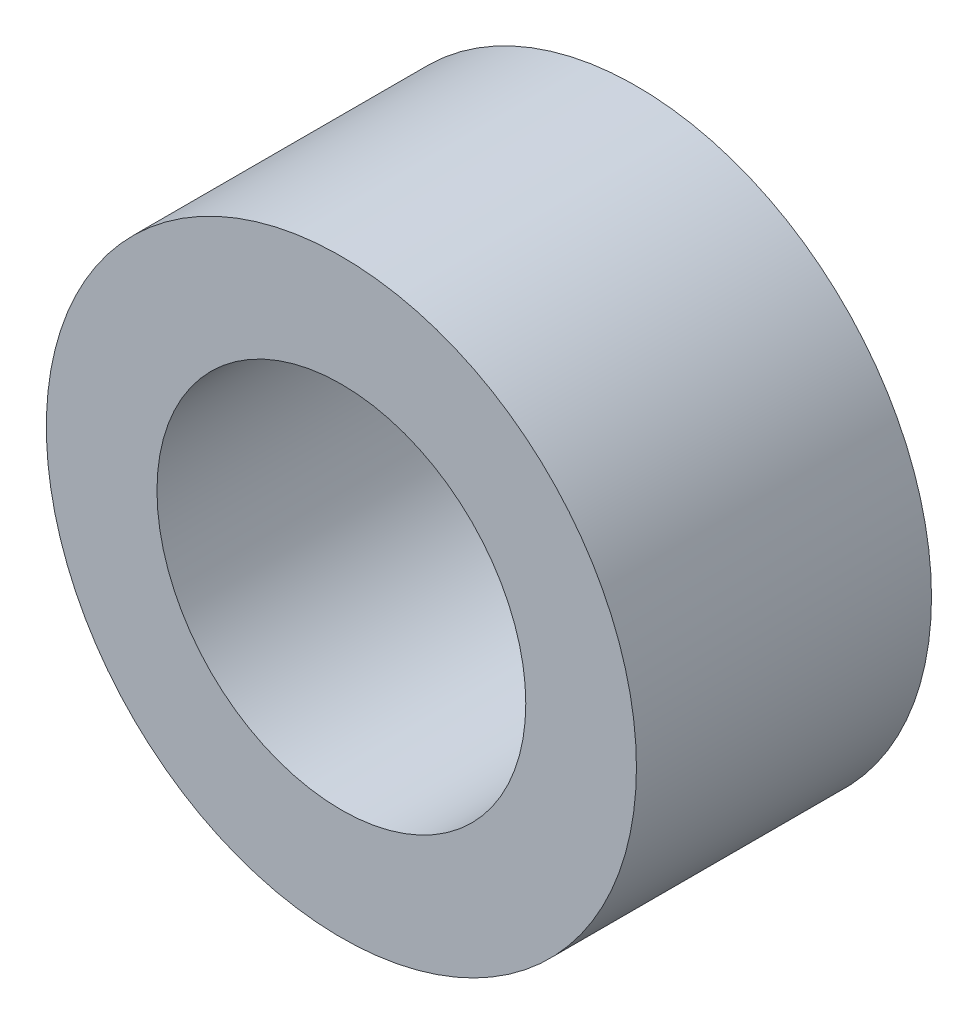
ISO-10303-21;
HEADER;
FILE_DESCRIPTION(('STEP AP214'),'2;1');
FILE_NAME('part.step','',(''),(''),'','','');
FILE_SCHEMA(('AUTOMOTIVE_DESIGN { 1 0 10303 214 1 1 1 1 }'));
ENDSEC;
DATA;
#1=APPLICATION_CONTEXT('core data for automotive mechanical design processes');
#2=APPLICATION_PROTOCOL_DEFINITION('international standard','automotive_design',2000,#1);
#3=PRODUCT_CONTEXT('',#1,'mechanical');
#4=PRODUCT('Part','Part','',(#3));
#5=PRODUCT_RELATED_PRODUCT_CATEGORY('part','',(#4));
#6=PRODUCT_DEFINITION_FORMATION('','',#4);
#7=PRODUCT_DEFINITION_CONTEXT('part definition',#1,'design');
#8=PRODUCT_DEFINITION('design','',#6,#7);
#9=PRODUCT_DEFINITION_SHAPE('','',#8);
#10=(LENGTH_UNIT() NAMED_UNIT(*) SI_UNIT(.MILLI.,.METRE.));
#11=(NAMED_UNIT(*) PLANE_ANGLE_UNIT() SI_UNIT($,.RADIAN.));
#12=(NAMED_UNIT(*) SI_UNIT($,.STERADIAN.) SOLID_ANGLE_UNIT());
#13=UNCERTAINTY_MEASURE_WITH_UNIT(LENGTH_MEASURE(1.E-05),#10,'distance_accuracy_value','');
#14=(GEOMETRIC_REPRESENTATION_CONTEXT(3) GLOBAL_UNCERTAINTY_ASSIGNED_CONTEXT((#13)) GLOBAL_UNIT_ASSIGNED_CONTEXT((#10,
#11,#12)) REPRESENTATION_CONTEXT('',''));
#15=CARTESIAN_POINT('',(0.,0.,0.));
#16=DIRECTION('',(0.,0.,1.));
#17=DIRECTION('',(1.,0.,0.));
#18=AXIS2_PLACEMENT_3D('',#15,#16,#17);
#19=CARTESIAN_POINT('',(0.,0.,2.5));
#20=DIRECTION('',(0.,0.,1.));
#21=DIRECTION('',(1.,0.,0.));
#22=AXIS2_PLACEMENT_3D('',#19,#20,#21);
#23=PLANE('',#22);
#24=CARTESIAN_POINT('',(0.,0.,2.5));
#25=DIRECTION('',(0.,0.,1.));
#26=DIRECTION('',(1.,0.,0.));
#27=AXIS2_PLACEMENT_3D('',#24,#25,#26);
#28=CIRCLE('',#27,5.);
#29=CARTESIAN_POINT('',(5.,0.,2.5));
#30=VERTEX_POINT('',#29);
#31=EDGE_CURVE('E10',#30,#30,#28,.T.);
#32=ORIENTED_EDGE('',*,*,#31,.T.);
#33=EDGE_LOOP('',(#32));
#34=FACE_BOUND('',#33,.T.);
#35=CARTESIAN_POINT('',(0.,0.,2.5));
#36=DIRECTION('',(0.,0.,1.));
#37=DIRECTION('',(1.,0.,0.));
#38=AXIS2_PLACEMENT_3D('',#35,#36,#37);
#39=CIRCLE('',#38,3.125);
#40=CARTESIAN_POINT('',(3.125,0.,2.5));
#41=VERTEX_POINT('',#40);
#42=EDGE_CURVE('E55',#41,#41,#39,.T.);
#43=ORIENTED_EDGE('',*,*,#42,.F.);
#44=EDGE_LOOP('',(#43));
#45=FACE_BOUND('',#44,.T.);
#46=ADVANCED_FACE('F41',(#34,#45),#23,.T.);
#47=CARTESIAN_POINT('',(0.,0.,-2.5));
#48=DIRECTION('',(0.,0.,1.));
#49=DIRECTION('',(1.,0.,0.));
#50=AXIS2_PLACEMENT_3D('',#47,#48,#49);
#51=PLANE('',#50);
#52=CARTESIAN_POINT('',(0.,0.,-2.5));
#53=DIRECTION('',(0.,0.,1.));
#54=DIRECTION('',(1.,0.,0.));
#55=AXIS2_PLACEMENT_3D('',#52,#53,#54);
#56=CIRCLE('',#55,5.);
#57=CARTESIAN_POINT('',(5.,0.,-2.5));
#58=VERTEX_POINT('',#57);
#59=EDGE_CURVE('E44',#58,#58,#56,.T.);
#60=ORIENTED_EDGE('',*,*,#59,.F.);
#61=EDGE_LOOP('',(#60));
#62=FACE_BOUND('',#61,.T.);
#63=CARTESIAN_POINT('',(0.,0.,-2.5));
#64=DIRECTION('',(0.,0.,1.));
#65=DIRECTION('',(1.,0.,0.));
#66=AXIS2_PLACEMENT_3D('',#63,#64,#65);
#67=CIRCLE('',#66,3.125);
#68=CARTESIAN_POINT('',(3.125,0.,-2.5));
#69=VERTEX_POINT('',#68);
#70=EDGE_CURVE('E53',#69,#69,#67,.T.);
#71=ORIENTED_EDGE('',*,*,#70,.T.);
#72=EDGE_LOOP('',(#71));
#73=FACE_BOUND('',#72,.T.);
#74=ADVANCED_FACE('F61',(#62,#73),#51,.F.);
#75=CARTESIAN_POINT('',(0.,0.,2.5));
#76=DIRECTION('',(0.,0.,-1.));
#77=DIRECTION('',(-1.,0.,0.));
#78=AXIS2_PLACEMENT_3D('',#75,#76,#77);
#79=CYLINDRICAL_SURFACE('',#78,5.);
#80=ORIENTED_EDGE('',*,*,#31,.F.);
#81=EDGE_LOOP('',(#80));
#82=FACE_BOUND('',#81,.T.);
#83=ORIENTED_EDGE('',*,*,#59,.T.);
#84=EDGE_LOOP('',(#83));
#85=FACE_BOUND('',#84,.T.);
#86=ADVANCED_FACE('F43',(#82,#85),#79,.T.);
#87=CARTESIAN_POINT('',(0.,0.,2.5));
#88=DIRECTION('',(0.,0.,-1.));
#89=DIRECTION('',(-1.,0.,0.));
#90=AXIS2_PLACEMENT_3D('',#87,#88,#89);
#91=CYLINDRICAL_SURFACE('',#90,3.125);
#92=ORIENTED_EDGE('',*,*,#42,.T.);
#93=EDGE_LOOP('',(#92));
#94=FACE_BOUND('',#93,.T.);
#95=ORIENTED_EDGE('',*,*,#70,.F.);
#96=EDGE_LOOP('',(#95));
#97=FACE_BOUND('',#96,.T.);
#98=ADVANCED_FACE('F58',(#94,#97),#91,.F.);
#99=CLOSED_SHELL('',(#46,#74,#86,#98));
#100=MANIFOLD_SOLID_BREP('B2',#99);
#101=ADVANCED_BREP_SHAPE_REPRESENTATION('',(#18,#100),#14);
#102=SHAPE_DEFINITION_REPRESENTATION(#9,#101);
ENDSEC;
END-ISO-10303-21;
